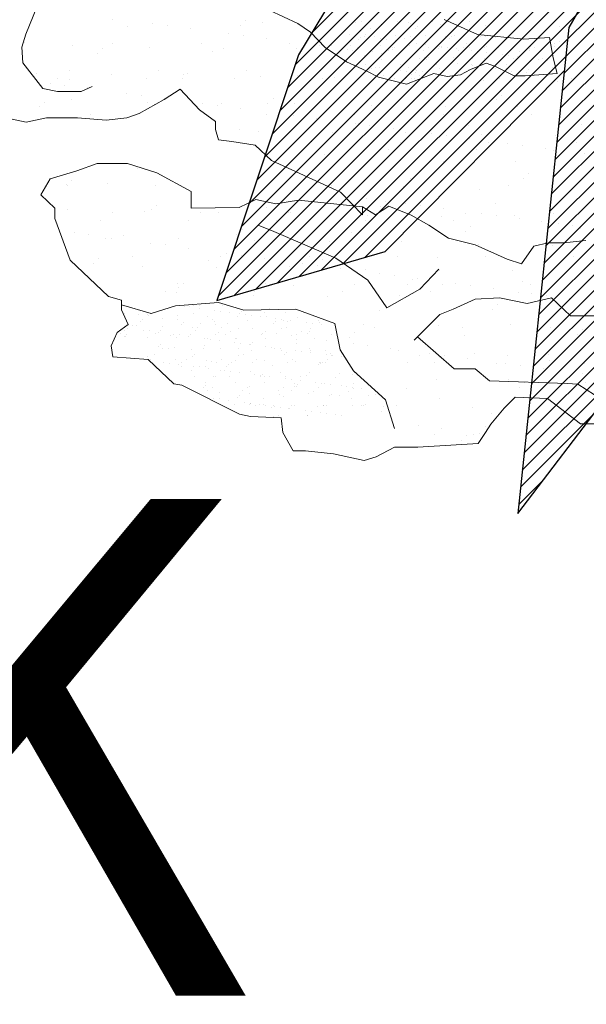
# Model space of a CAD drawing. Units: inches. Extents: x 1986 to 21484, y -1816 to 2016.
# Tile 12 of 85: x 2157 to 2165, y 1860 to 1874. Entities that reach past the tile are written whole.
import ezdxf

# ---------------------------------------------------------------- set-up
doc = ezdxf.new("R2010")
doc.units = ezdxf.units.IN
for name, color, linetype, lineweight in [('A-ANNO-TEXT', 7, 'Continuous', 18), ('L-PLNT', 84, 'Continuous', 13), ('vfolhas', 114, 'Continuous', 5)]:
    doc.layers.add(name, color=color, linetype=linetype, lineweight=lineweight)
doc.layers.add('vfolha2', color=110, linetype='Continuous')
doc.layers.add('vfolhas2', color=102, linetype='Continuous')
doc.styles.get("Standard").update_dxf_attribs({"font": 'arial.ttf'})
pattern_1 = [(45, (-2446.5133113, 50.986076), (-0.004419417382, 0.004419417382), [])]

# ---------------------------------------------------------------- blocks, each defined once
blk = doc.blocks.new('arbusto_PB_verde_grande')
at = {"layer": 'vfolha2'}
h = blk.add_hatch(dxfattribs=at)
h.set_pattern_fill('ANSI31', color=256, scale=0.05, style=0)
h.set_pattern_definition(pattern_1)
h.paths.add_polyline_path([(0.02944, 0.35651), (0.00028, 0.09048), (0.02625, -0.03934), (0.047, 0.06233), (0.06189, 0.09731), (0.09372, 0.26573), (0.09955, 0.43473), (0.08789, 0.61313), (0.0645, 0.72266), (0.04988, 0.6851), (0.0236, 0.51294)])
h.paths.add_polyline_path([(0.30106, 0.43789), (0.14225, 0.24871), (0.26685, 0.30022)])
h.paths.add_polyline_path([(0.37995, 0.22817), (0.23697, 0.15193), (0.18428, 0.09364), (0.11122, 0.04358), (0.02625, -0.03934), (0.28061, 0.04667), (0.36829, 0.07798), (0.46756, 0.11239), (0.61068, 0.19376), (0.71585, 0.27823), (0.55813, 0.25948)])
h.paths.add_polyline_path([(0.56101, -0.29441), (0.72752, -0.32573), (0.59024, -0.2412), (0.42962, -0.15982), (0.02625, -0.03934), (0.14922, -0.14107), (0.18838, -0.16604), (0.41501, -0.24435)])
h.paths.add_polyline_path([(-0.27429, -0.44776), (-0.30352, -0.72628), (-0.23923, -0.64175), (-0.15457, -0.45716), (0.02625, -0.03934), (-0.16328, -0.25376)])
h.paths.add_polyline_path([(-0.51963, -0.24744), (-0.67736, -0.32573), (-0.59558, -0.35072), (-0.40574, -0.32882), (-0.21007, -0.20995), (0.02625, -0.03934), (-0.14874, -0.06595), (-0.31518, -0.09101), (-0.41452, -0.15048)])
h.paths.add_polyline_path([(-0.52546, 0.25007), (-0.70947, 0.24698), (-0.51963, 0.1093), (-0.32979, 0.02167), (-0.07567, -0.0128), (-0.04234, -0.02148), (-0.35024, 0.1312)])
at = {"layer": 'vfolhas'}
h = blk.add_hatch(dxfattribs=at)
h.set_pattern_fill('ANSI31', color=256, scale=0.05, style=0)
h.set_pattern_definition(pattern_1)
h.paths.add_polyline_path([(-0.57219, 0.06233), (-0.7153, 0.10298), (-0.67736, 0.08107), (-0.62769, 0.01536), (-0.56347, -0.04095), (-0.26461, -0.0834), (-0.14874, -0.06595), (-0.10151, -0.05877), (-0.20418, -0.0472), (-0.40279, -0.00339)])
h.paths.add_polyline_path([(-0.56347, -0.04095), (-0.58279, -0.02401), (-0.72992, -0.09726), (-0.4334, -0.1679), (-0.41452, -0.15048), (-0.31518, -0.09101), (-0.26461, -0.0834)])
h.paths.add_polyline_path([(-0.2769, -0.47267), (-0.27429, -0.44776), (-0.16328, -0.25376), (0.02625, -0.03934), (-0.21007, -0.20995), (-0.2672, -0.24466), (-0.36485, -0.35697), (-0.42907, -0.46341), (-0.47586, -0.60425), (-0.37946, -0.57603)])
at = {"layer": 'vfolha2'}
for p, q in [((-0.16328, -0.25376), (-0.27429, -0.44776)), ((-0.27429, -0.44776), (-0.30352, -0.72628)), ((-0.30352, -0.72628), (-0.23923, -0.64175))]:
    blk.add_line(p, q, dxfattribs=at)
at = {"layer": 'vfolhas2'}
for p, q in [((-0.36485, -0.35697), (-0.42907, -0.46341)), ((-0.42907, -0.46341), (-0.47586, -0.60425)), ((-0.37946, -0.57603), (-0.2769, -0.47267)), ((-0.47586, -0.60425), (-0.37946, -0.57603))]:
    blk.add_line(p, q, dxfattribs=at)
blk = doc.blocks.new('PLANT-SHRUB')
for p, q in [((2157.221, 1873.694), (2157.486, 1874.349)), ((2161.057, 1873.846), (2160.649, 1874.033)), ((2158.449, 1873.897), (2158.449, 1873.897)), ((2158.651, 1873.807), (2158.651, 1873.807)), ((2159.005, 1873.85), (2159.005, 1873.85)), ((2159.213, 1873.823), (2159.213, 1873.823)), ((2160.25, 1873.821), (2160.25, 1873.821)), ((2160.324, 1873.889), (2160.324, 1873.889)), ((2160.551, 1873.863), (2160.551, 1873.863)), ((2161.233, 1873.725), (2161.057, 1873.846)), ((2161.597, 1873.849), (2161.597, 1873.849)), ((2161.873, 1873.857), (2161.873, 1873.857)), ((2161.959, 1873.87), (2161.959, 1873.87)), ((2162.228, 1873.838), (2162.228, 1873.838)), ((2162.457, 1873.869), (2162.457, 1873.869)), ((2162.619, 1873.854), (2162.619, 1873.854)), ((2162.637, 1873.84), (2162.637, 1873.84)), ((2162.748, 1873.808), (2162.748, 1873.808)), ((2162.955, 1873.868), (2162.955, 1873.868)), ((2163.069, 1873.825), (2163.069, 1873.825)), ((2163.116, 1873.901), (2163.589, 1873.692)), ((2163.472, 1873.87), (2163.472, 1873.87)), ((2163.699, 1873.815), (2163.699, 1873.815)), ((2164.745, 1873.802), (2164.745, 1873.802)), ((2157.166, 1873.513), (2157.221, 1873.694)), ((2159.538, 1873.78), (2159.538, 1873.78)), ((2160.081, 1873.709), (2160.081, 1873.709)), ((2160.289, 1873.681), (2160.289, 1873.681)), ((2161.442, 1873.505), (2161.233, 1873.725)), ((2161.786, 1873.691), (2161.786, 1873.691)), ((2161.869, 1873.68), (2161.869, 1873.68)), ((2161.999, 1873.663), (2161.999, 1873.663)), ((2162.003, 1873.696), (2162.003, 1873.696)), ((2162.079, 1873.775), (2162.079, 1873.775)), ((2162.14, 1873.667), (2162.14, 1873.667)), ((2162.434, 1873.68), (2162.434, 1873.68)), ((2162.638, 1873.666), (2162.638, 1873.666)), ((2162.718, 1873.781), (2162.718, 1873.781)), ((2162.853, 1873.675), (2162.853, 1873.675)), ((2163.136, 1873.665), (2163.136, 1873.665)), ((2163.228, 1873.667), (2163.228, 1873.667)), ((2163.262, 1873.677), (2163.262, 1873.677)), ((2163.589, 1873.692), (2164.239, 1873.626)), ((2163.634, 1873.664), (2163.634, 1873.664)), ((2163.694, 1873.661), (2163.694, 1873.661)), ((2163.848, 1873.654), (2163.848, 1873.654)), ((2157.18, 1873.29), (2157.166, 1873.513)), ((2157.203, 1873.572), (2157.203, 1873.572)), ((2157.885, 1873.54), (2157.885, 1873.54)), ((2158.447, 1873.57), (2158.447, 1873.57)), ((2159.692, 1873.568), (2159.692, 1873.568)), ((2160.614, 1873.639), (2160.614, 1873.639)), ((2160.937, 1873.565), (2160.937, 1873.565)), ((2161.157, 1873.567), (2161.157, 1873.567)), ((2161.365, 1873.54), (2161.365, 1873.54)), ((2161.525, 1873.538), (2161.525, 1873.538)), ((2161.8, 1873.536), (2161.8, 1873.536)), ((2161.897, 1873.512), (2161.897, 1873.512)), ((2161.91, 1873.621), (2161.91, 1873.621)), ((2161.94, 1873.648), (2161.94, 1873.648)), ((2162.181, 1873.563), (2162.181, 1873.563)), ((2162.216, 1873.635), (2162.216, 1873.635)), ((2162.218, 1873.53), (2162.218, 1873.53)), ((2162.299, 1873.624), (2162.299, 1873.624)), ((2162.395, 1873.512), (2162.395, 1873.512)), ((2162.429, 1873.607), (2162.429, 1873.607)), ((2162.559, 1873.635), (2162.559, 1873.635)), ((2162.627, 1873.532), (2162.627, 1873.532)), ((2162.646, 1873.578), (2162.646, 1873.578)), ((2162.73, 1873.567), (2162.73, 1873.567)), ((2162.86, 1873.55), (2162.86, 1873.55)), ((2163.059, 1873.517), (2163.059, 1873.517)), ((2163.077, 1873.521), (2163.077, 1873.521)), ((2163.199, 1873.64), (2163.199, 1873.64)), ((2163.426, 1873.561), (2163.426, 1873.561)), ((2163.477, 1873.511), (2163.477, 1873.511)), ((2163.709, 1873.527), (2163.709, 1873.527)), ((2163.886, 1873.513), (2163.886, 1873.513)), ((2164.239, 1873.626), (2164.602, 1873.648)), ((2164.329, 1873.514), (2164.329, 1873.514)), ((2164.602, 1873.648), (2164.657, 1873.362)), ((2164.602, 1873.648), (2164.602, 1873.648)), ((2164.671, 1873.559), (2164.671, 1873.559)), ((2164.673, 1873.52), (2164.673, 1873.52)), ((2164.747, 1873.587), (2164.747, 1873.587)), ((2158.229, 1873.421), (2158.229, 1873.421)), ((2158.303, 1873.489), (2158.303, 1873.489)), ((2158.964, 1873.501), (2158.964, 1873.501)), ((2159.852, 1873.457), (2159.852, 1873.457)), ((2160.01, 1873.488), (2160.01, 1873.488)), ((2161.033, 1873.493), (2161.033, 1873.493)), ((2161.739, 1873.307), (2161.442, 1873.505)), ((2161.451, 1873.47), (2161.451, 1873.47)), ((2161.69, 1873.497), (2161.69, 1873.497)), ((2161.751, 1873.475), (2161.751, 1873.475)), ((2161.83, 1873.47), (2161.83, 1873.47)), ((2161.993, 1873.388), (2161.993, 1873.388)), ((2162.112, 1873.454), (2162.112, 1873.454)), ((2162.233, 1873.426), (2162.233, 1873.426)), ((2162.328, 1873.469), (2162.328, 1873.469)), ((2162.391, 1873.48), (2162.391, 1873.48)), ((2162.42, 1873.507), (2162.42, 1873.507)), ((2162.424, 1873.372), (2162.424, 1873.372)), ((2162.441, 1873.398), (2162.441, 1873.398)), ((2162.826, 1873.468), (2162.826, 1873.468)), ((2162.893, 1873.511), (2162.893, 1873.511)), ((2163.04, 1873.494), (2163.04, 1873.494)), ((2163.074, 1873.506), (2163.074, 1873.506)), ((2163.158, 1873.441), (2163.158, 1873.441)), ((2163.16, 1873.51), (2163.16, 1873.51)), ((2163.29, 1873.493), (2163.29, 1873.493)), ((2163.324, 1873.467), (2163.324, 1873.467)), ((2163.391, 1873.51), (2163.391, 1873.51)), ((2163.507, 1873.465), (2163.507, 1873.465)), ((2163.59, 1873.454), (2163.59, 1873.454)), ((2163.68, 1873.5), (2163.68, 1873.5)), ((2163.72, 1873.437), (2163.72, 1873.437)), ((2163.821, 1873.466), (2163.821, 1873.466)), ((2163.889, 1873.509), (2163.889, 1873.509)), ((2163.937, 1873.408), (2163.937, 1873.408)), ((2164.021, 1873.397), (2164.021, 1873.397)), ((2164.151, 1873.38), (2164.151, 1873.38)), ((2164.181, 1873.446), (2164.181, 1873.446)), ((2164.19, 1873.387), (2164.19, 1873.387)), ((2164.318, 1873.498), (2164.318, 1873.498)), ((2164.319, 1873.465), (2164.319, 1873.465)), ((2164.387, 1873.508), (2164.387, 1873.508)), ((2157.458, 1872.928), (2157.18, 1873.29)), ((2162.026, 1873.175), (2161.739, 1873.307)), ((2161.851, 1873.269), (2161.851, 1873.269)), ((2162.011, 1873.267), (2162.011, 1873.267)), ((2162.069, 1873.24), (2162.069, 1873.24)), ((2162.232, 1873.334), (2162.232, 1873.334)), ((2162.509, 1873.266), (2162.509, 1873.266)), ((2162.766, 1873.355), (2162.766, 1873.355)), ((2162.843, 1873.367), (2162.843, 1873.367)), ((2162.871, 1873.34), (2162.871, 1873.34)), ((2162.901, 1873.367), (2162.901, 1873.367)), ((2163.007, 1873.265), (2163.007, 1873.265)), ((2163.252, 1873.369), (2163.252, 1873.369)), ((2163.308, 1873.284), (2163.308, 1873.284)), ((2163.71, 1873.285), (2163.49, 1873.197)), ((2163.505, 1873.264), (2163.505, 1873.264)), ((2163.517, 1873.257), (2163.517, 1873.257)), ((2163.52, 1873.354), (2163.52, 1873.354)), ((2163.684, 1873.353), (2163.684, 1873.353)), ((2163.842, 1873.241), (2163.71, 1873.285)), ((2164.107, 1873.109), (2163.842, 1873.241)), ((2164.002, 1873.263), (2164.002, 1873.263)), ((2164.102, 1873.348), (2164.102, 1873.348)), ((2164.16, 1873.36), (2164.16, 1873.36)), ((2164.368, 1873.351), (2164.368, 1873.351)), ((2164.451, 1873.34), (2164.451, 1873.34)), ((2164.5, 1873.262), (2164.5, 1873.262)), ((2164.511, 1873.35), (2164.511, 1873.35)), ((2164.581, 1873.323), (2164.581, 1873.323)), ((2164.657, 1873.362), (2164.712, 1873.142)), ((2164.67, 1873.246), (2164.67, 1873.246)), ((2157.377, 1873.14), (2157.377, 1873.14)), ((2157.841, 1873.183), (2157.841, 1873.183)), ((2158.424, 1873.127), (2158.424, 1873.127)), ((2159.085, 1873.181), (2159.085, 1873.181)), ((2159.446, 1873.132), (2159.446, 1873.132)), ((2159.504, 1873.138), (2159.504, 1873.138)), ((2160.33, 1873.179), (2160.33, 1873.179)), ((2161.054, 1873.106), (2161.054, 1873.106)), ((2161.575, 1873.177), (2161.575, 1873.177)), ((2162.191, 1873.087), (2162.026, 1873.175)), ((2162.063, 1873.18), (2162.063, 1873.18)), ((2162.092, 1873.207), (2162.092, 1873.207)), ((2162.152, 1873.229), (2162.152, 1873.229)), ((2162.208, 1873.222), (2162.208, 1873.222)), ((2162.266, 1873.111), (2162.266, 1873.111)), ((2162.282, 1873.212), (2162.282, 1873.212)), ((2162.499, 1873.184), (2162.499, 1873.184)), ((2162.582, 1873.173), (2162.582, 1873.173)), ((2162.973, 1873.142), (2162.587, 1872.988)), ((2162.617, 1873.224), (2162.617, 1873.224)), ((2162.653, 1873.12), (2162.653, 1873.12)), ((2162.712, 1873.194), (2162.712, 1873.194)), ((2162.712, 1873.155), (2162.712, 1873.155)), ((2162.726, 1873.187), (2162.726, 1873.187)), ((2162.764, 1873.11), (2162.764, 1873.11)), ((2162.819, 1873.174), (2162.819, 1873.174)), ((2162.929, 1873.127), (2162.929, 1873.127)), ((2162.973, 1873.142), (2162.973, 1873.142)), ((2163.16, 1873.098), (2162.973, 1873.142)), ((2163.049, 1873.209), (2163.049, 1873.209)), ((2163.347, 1873.12), (2163.16, 1873.098)), ((2163.49, 1873.197), (2163.347, 1873.12)), ((2163.352, 1873.2), (2163.352, 1873.2)), ((2163.381, 1873.227), (2163.381, 1873.227)), ((2163.467, 1873.203), (2163.467, 1873.203)), ((2163.841, 1873.214), (2163.841, 1873.214)), ((2164.001, 1873.214), (2164.001, 1873.214)), ((2164.064, 1873.172), (2164.064, 1873.172)), ((2164.261, 1873.109), (2164.107, 1873.109)), ((2164.712, 1873.142), (2164.261, 1873.109)), ((2164.276, 1873.155), (2164.276, 1873.155)), ((2164.308, 1873.19), (2164.308, 1873.19)), ((2164.384, 1873.142), (2164.384, 1873.142)), ((2164.592, 1873.115), (2164.592, 1873.115)), ((2164.641, 1873.219), (2164.641, 1873.219)), ((2164.712, 1873.142), (2164.712, 1873.142)), ((2157.561, 1873.006), (2157.561, 1873.006)), ((2157.672, 1873.076), (2157.672, 1873.076)), ((2157.769, 1872.978), (2157.769, 1872.978)), ((2157.831, 1873.057), (2157.831, 1873.057)), ((2158.155, 1872.956), (2158.002, 1872.886)), ((2158.917, 1873.074), (2158.917, 1873.074)), ((2159.431, 1873.071), (2159.431, 1873.071)), ((2160.161, 1873.071), (2160.161, 1873.071)), ((2160.525, 1873.093), (2160.525, 1873.093)), ((2161.406, 1873.069), (2161.406, 1873.069)), ((2161.572, 1873.079), (2161.572, 1873.079)), ((2162.587, 1872.988), (2162.191, 1873.087)), ((2162.414, 1873.064), (2162.414, 1873.064)), ((2162.544, 1873.04), (2162.544, 1873.04)), ((2162.573, 1873.067), (2162.573, 1873.067)), ((2162.594, 1873.084), (2162.594, 1873.084)), ((2162.651, 1873.067), (2162.651, 1873.067)), ((2162.697, 1873.067), (2162.697, 1873.067)), ((2163.673, 1873.045), (2163.673, 1873.045)), ((2163.895, 1873.065), (2163.895, 1873.065)), ((2164.72, 1873.032), (2164.72, 1873.032)), ((2164.917, 1873.072), (2164.917, 1873.072)), ((2157.458, 1872.928), (2157.458, 1872.928)), ((2157.667, 1872.886), (2157.458, 1872.928)), ((2157.667, 1872.886), (2157.667, 1872.886)), ((2158.002, 1872.886), (2157.667, 1872.886)), ((2158.002, 1872.886), (2158.002, 1872.886)), ((2158.094, 1872.936), (2158.094, 1872.936)), ((2158.637, 1872.864), (2158.637, 1872.864)), ((2158.845, 1872.837), (2158.845, 1872.837)), ((2159.398, 1872.918), (2159.17, 1872.773)), ((2159.667, 1872.628), (2159.398, 1872.918)), ((2163.928, 1872.836), (2163.928, 1872.836)), ((2157.484, 1872.738), (2157.484, 1872.738)), ((2157.859, 1872.77), (2157.859, 1872.77)), ((2159.17, 1872.773), (2158.818, 1872.576)), ((2158.939, 1872.731), (2158.939, 1872.731)), ((2159.033, 1872.706), (2159.033, 1872.706)), ((2159.17, 1872.794), (2159.17, 1872.794)), ((2159.713, 1872.723), (2159.713, 1872.723)), ((2159.921, 1872.695), (2159.921, 1872.695)), ((2159.985, 1872.718), (2159.985, 1872.718)), ((2160.632, 1872.72), (2160.632, 1872.72)), ((2160.706, 1872.787), (2160.706, 1872.787)), ((2161.007, 1872.723), (2161.007, 1872.723)), ((2162.087, 1872.684), (2162.087, 1872.684)), ((2162.255, 1872.755), (2162.255, 1872.755)), ((2163.854, 1872.769), (2163.854, 1872.769)), ((2157.223, 1872.452), (2156.653, 1872.576)), ((2157.41, 1872.671), (2157.41, 1872.671)), ((2158.125, 1872.569), (2158.125, 1872.569)), ((2158.818, 1872.576), (2158.642, 1872.514)), ((2159.895, 1872.463), (2159.667, 1872.628)), ((2160.245, 1872.652), (2160.245, 1872.652)), ((2160.614, 1872.565), (2160.614, 1872.565)), ((2160.788, 1872.581), (2160.788, 1872.581)), ((2160.996, 1872.554), (2160.996, 1872.554)), ((2161.858, 1872.562), (2161.858, 1872.562)), ((2163.103, 1872.56), (2163.103, 1872.56)), ((2163.133, 1872.671), (2163.133, 1872.671)), ((2164.155, 1872.675), (2164.155, 1872.675)), ((2164.348, 1872.558), (2164.348, 1872.558)), ((2157.513, 1872.514), (2157.223, 1872.452)), ((2157.223, 1872.452), (2157.223, 1872.452)), ((2157.948, 1872.514), (2157.513, 1872.514)), ((2158.352, 1872.483), (2157.948, 1872.514)), ((2158.642, 1872.514), (2158.352, 1872.483)), ((2159.895, 1872.349), (2159.895, 1872.463)), ((2161.321, 1872.511), (2161.321, 1872.511)), ((2161.864, 1872.439), (2161.864, 1872.439)), ((2161.907, 1872.437), (2161.907, 1872.437)), ((2162.072, 1872.412), (2162.072, 1872.412)), ((2163.456, 1872.404), (2163.456, 1872.404)), ((2165.056, 1872.418), (2165.056, 1872.418)), ((2159.936, 1872.204), (2159.895, 1872.349)), ((2160.234, 1872.355), (2160.234, 1872.355)), ((2160.5, 1872.323), (2160.5, 1872.323)), ((2161.546, 1872.309), (2161.546, 1872.309)), ((2161.834, 1872.369), (2161.834, 1872.369)), ((2162.397, 1872.369), (2162.397, 1872.369)), ((2162.569, 1872.314), (2162.569, 1872.314)), ((2162.94, 1872.298), (2162.94, 1872.298)), ((2163.148, 1872.27), (2163.148, 1872.27)), ((2163.648, 1872.275), (2163.648, 1872.275)), ((2164.694, 1872.262), (2164.694, 1872.262)), ((2160.123, 1872.183), (2159.936, 1872.204)), ((2160.454, 1872.131), (2160.123, 1872.183)), ((2160.682, 1871.914), (2160.454, 1872.131)), ((2161.252, 1872.176), (2161.252, 1872.176)), ((2162.496, 1872.173), (2162.496, 1872.173)), ((2163.473, 1872.227), (2163.473, 1872.227)), ((2163.741, 1872.171), (2163.741, 1872.171)), ((2164.016, 1872.156), (2164.016, 1872.156)), ((2164.224, 1872.129), (2164.224, 1872.129)), ((2164.986, 1872.169), (2164.986, 1872.169)), ((2161.436, 1872.005), (2161.436, 1872.005)), ((2162.328, 1872.066), (2162.328, 1872.066)), ((2163.035, 1872.018), (2163.035, 1872.018)), ((2163.109, 1872.086), (2163.109, 1872.086)), ((2163.572, 1872.064), (2163.572, 1872.064)), ((2164.549, 1872.086), (2164.549, 1872.086)), ((2164.658, 1872.054), (2164.658, 1872.054)), ((2164.817, 1872.062), (2164.817, 1872.062)), ((2165.092, 1872.014), (2165.092, 1872.014)), ((2157.937, 1871.769), (2158.227, 1871.873)), ((2158.227, 1871.873), (2158.652, 1871.873)), ((2158.227, 1871.873), (2158.227, 1871.873)), ((2158.652, 1871.873), (2159.066, 1871.738)), ((2160.682, 1871.914), (2160.682, 1871.914)), ((2161.656, 1871.469), (2160.682, 1871.914)), ((2162.062, 1871.914), (2162.062, 1871.914)), ((2163.108, 1871.9), (2163.108, 1871.9)), ((2164.13, 1871.905), (2164.13, 1871.905)), ((2157.565, 1871.655), (2157.937, 1871.769)), ((2158.801, 1871.808), (2158.801, 1871.808)), ((2159.066, 1871.738), (2159.553, 1871.479)), ((2164.31, 1871.735), (2164.31, 1871.735)), ((2157.43, 1871.428), (2157.565, 1871.655)), ((2157.792, 1871.569), (2157.792, 1871.569)), ((2157.802, 1871.568), (2157.802, 1871.568)), ((2157.866, 1871.637), (2157.866, 1871.637)), ((2158.373, 1871.586), (2158.373, 1871.586)), ((2162.637, 1871.654), (2162.637, 1871.654)), ((2164.237, 1871.667), (2164.237, 1871.667)), ((2159.046, 1871.566), (2159.046, 1871.566)), ((2159.553, 1871.479), (2159.553, 1871.241)), ((2161.536, 1871.561), (2161.536, 1871.561)), ((2161.966, 1871.148), (2161.656, 1871.469)), ((2162.544, 1871.544), (2162.544, 1871.544)), ((2162.78, 1871.559), (2162.78, 1871.559)), ((2163.623, 1871.505), (2163.623, 1871.505)), ((2164.025, 1871.557), (2164.025, 1871.557)), ((2164.669, 1871.492), (2164.669, 1871.492)), ((2157.43, 1871.428), (2157.43, 1871.428)), ((2157.627, 1871.241), (2157.43, 1871.428)), ((2160.226, 1871.252), (2160.465, 1871.366)), ((2160.465, 1871.366), (2160.744, 1871.303)), ((2160.744, 1871.303), (2161.065, 1871.355)), ((2161.065, 1871.355), (2161.966, 1871.262)), ((2161.704, 1871.426), (2161.704, 1871.426)), ((2162.029, 1871.383), (2162.029, 1871.383)), ((2162.29, 1871.335), (2162.29, 1871.335)), ((2162.571, 1871.311), (2162.571, 1871.311)), ((2163.839, 1871.303), (2163.839, 1871.303)), ((2157.627, 1871.096), (2157.627, 1871.241)), ((2157.809, 1871.23), (2157.809, 1871.23)), ((2158.44, 1871.179), (2158.44, 1871.179)), ((2158.888, 1871.191), (2158.888, 1871.191)), ((2158.994, 1871.219), (2158.994, 1871.219)), ((2159.067, 1871.286), (2159.067, 1871.286)), ((2159.553, 1871.241), (2160.226, 1871.252)), ((2159.684, 1871.177), (2159.684, 1871.177)), ((2159.935, 1871.178), (2159.935, 1871.178)), ((2160.617, 1871.254), (2160.617, 1871.254)), ((2160.929, 1871.175), (2160.929, 1871.175)), ((2160.957, 1871.183), (2160.957, 1871.183)), ((2161.966, 1871.262), (2162.152, 1871.148)), ((2161.966, 1871.262), (2161.966, 1871.148)), ((2162.152, 1871.148), (2162.339, 1871.269)), ((2162.174, 1871.173), (2162.174, 1871.173)), ((2162.216, 1871.268), (2162.216, 1871.268)), ((2162.339, 1871.269), (2162.651, 1871.144)), ((2162.78, 1871.284), (2162.78, 1871.284)), ((2163.104, 1871.241), (2163.104, 1871.241)), ((2163.418, 1871.17), (2163.418, 1871.17)), ((2163.647, 1871.17), (2163.647, 1871.17)), ((2164.663, 1871.168), (2164.663, 1871.168)), ((2157.844, 1870.507), (2157.627, 1871.096)), ((2158.271, 1871.072), (2158.271, 1871.072)), ((2159.516, 1871.07), (2159.516, 1871.07)), ((2160.76, 1871.068), (2160.76, 1871.068)), ((2162.005, 1871.065), (2162.005, 1871.065)), ((2162.036, 1871.144), (2162.036, 1871.144)), ((2162.651, 1871.144), (2162.9, 1871.004)), ((2163.083, 1871.13), (2163.083, 1871.13)), ((2163.25, 1871.063), (2163.25, 1871.063)), ((2163.855, 1871.142), (2163.855, 1871.142)), ((2164.105, 1871.135), (2164.105, 1871.135)), ((2164.18, 1871.1), (2164.18, 1871.1)), ((2164.494, 1871.061), (2164.494, 1871.061)), ((2164.723, 1871.028), (2164.723, 1871.028)), ((2157.9, 1870.892), (2157.9, 1870.892)), ((2160.269, 1870.935), (2160.269, 1870.935)), ((2160.498, 1871.004), (2160.717, 1870.911)), ((2160.717, 1870.911), (2161.59, 1870.537)), ((2161.818, 1870.903), (2161.818, 1870.903)), ((2162.9, 1871.004), (2163.181, 1870.817)), ((2163.417, 1870.917), (2163.417, 1870.917)), ((2163.491, 1870.984), (2163.491, 1870.984)), ((2164.931, 1871.001), (2164.931, 1871.001)), ((2165.04, 1870.952), (2165.04, 1870.952)), ((2158.108, 1870.864), (2158.108, 1870.864)), ((2158.348, 1870.816), (2158.348, 1870.816)), ((2158.433, 1870.821), (2158.433, 1870.821)), ((2158.596, 1870.854), (2158.596, 1870.854)), ((2158.976, 1870.75), (2158.976, 1870.75)), ((2159.37, 1870.821), (2159.37, 1870.821)), ((2160.195, 1870.868), (2160.195, 1870.868)), ((2160.45, 1870.782), (2160.45, 1870.782)), ((2161.496, 1870.769), (2161.496, 1870.769)), ((2162.518, 1870.774), (2162.518, 1870.774)), ((2163.181, 1870.817), (2163.555, 1870.724)), ((2163.181, 1870.817), (2163.181, 1870.817)), ((2163.598, 1870.735), (2163.598, 1870.735)), ((2164.382, 1870.708), (2164.585, 1870.755)), ((2164.585, 1870.755), (2164.803, 1870.755)), ((2164.803, 1870.755), (2165.115, 1870.786)), ((2165.115, 1870.786), (2165.115, 1870.786)), ((2159.184, 1870.723), (2159.184, 1870.723)), ((2159.508, 1870.68), (2159.508, 1870.68)), ((2160.051, 1870.608), (2160.051, 1870.608)), ((2163.555, 1870.724), (2164.008, 1870.521)), ((2164.21, 1870.459), (2164.382, 1870.708)), ((2164.644, 1870.722), (2164.644, 1870.722)), ((2164.692, 1870.634), (2164.692, 1870.634)), ((2157.844, 1870.507), (2157.844, 1870.507)), ((2158.384, 1869.997), (2157.844, 1870.507)), ((2158.175, 1870.468), (2158.175, 1870.468)), ((2158.248, 1870.535), (2158.248, 1870.535)), ((2158.724, 1870.565), (2158.724, 1870.565)), ((2159.797, 1870.503), (2159.797, 1870.503)), ((2159.968, 1870.563), (2159.968, 1870.563)), ((2160.259, 1870.581), (2160.259, 1870.581)), ((2160.584, 1870.538), (2160.584, 1870.538)), ((2161.127, 1870.467), (2161.127, 1870.467)), ((2161.213, 1870.561), (2161.213, 1870.561)), ((2161.397, 1870.517), (2161.397, 1870.517)), ((2161.47, 1870.584), (2161.47, 1870.584)), ((2161.59, 1870.537), (2162.042, 1870.225)), ((2162.458, 1870.558), (2162.458, 1870.558)), ((2163.02, 1870.552), (2163.02, 1870.552)), ((2163.702, 1870.556), (2163.702, 1870.556)), ((2164.008, 1870.521), (2164.21, 1870.459)), ((2164.619, 1870.566), (2164.619, 1870.566)), ((2164.947, 1870.554), (2164.947, 1870.554)), ((2158.863, 1870.421), (2158.863, 1870.421)), ((2159.909, 1870.408), (2159.909, 1870.408)), ((2160.932, 1870.413), (2160.932, 1870.413)), ((2161.335, 1870.439), (2161.335, 1870.439)), ((2161.66, 1870.396), (2161.66, 1870.396)), ((2162.011, 1870.374), (2162.011, 1870.374)), ((2162.203, 1870.325), (2162.203, 1870.325)), ((2162.775, 1870.1), (2163.041, 1870.381)), ((2163.057, 1870.36), (2163.057, 1870.36)), ((2164.08, 1870.365), (2164.08, 1870.365)), ((2159.45, 1870.185), (2159.45, 1870.185)), ((2162.042, 1870.225), (2162.308, 1869.835)), ((2162.411, 1870.298), (2162.411, 1870.298)), ((2162.672, 1870.234), (2162.672, 1870.234)), ((2162.736, 1870.255), (2162.736, 1870.255)), ((2163.279, 1870.183), (2163.279, 1870.183)), ((2164.221, 1870.202), (2164.221, 1870.202)), ((2158.323, 1870.046), (2158.323, 1870.046)), ((2159.193, 1870.069), (2159.193, 1870.069)), ((2159.345, 1870.051), (2159.345, 1870.051)), ((2159.362, 1870.176), (2159.362, 1870.176)), ((2159.376, 1870.117), (2159.376, 1870.117)), ((2160.438, 1870.067), (2160.438, 1870.067)), ((2160.606, 1870.174), (2160.606, 1870.174)), ((2160.999, 1870.152), (2160.999, 1870.152)), ((2161.682, 1870.064), (2161.682, 1870.064)), ((2161.851, 1870.172), (2161.851, 1870.172)), ((2162.308, 1869.835), (2162.775, 1870.1)), ((2162.598, 1870.166), (2162.598, 1870.166)), ((2162.927, 1870.062), (2162.927, 1870.062)), ((2163.095, 1870.17), (2163.095, 1870.17)), ((2163.487, 1870.156), (2163.487, 1870.156)), ((2163.812, 1870.113), (2163.812, 1870.113)), ((2164.172, 1870.06), (2164.172, 1870.06)), ((2164.34, 1870.167), (2164.34, 1870.167)), ((2164.355, 1870.042), (2164.355, 1870.042)), ((2158.384, 1869.997), (2158.384, 1869.997)), ((2158.57, 1869.945), (2158.384, 1869.997)), ((2158.57, 1869.81), (2158.57, 1869.945)), ((2159.329, 1869.866), (2159.937, 1869.913)), ((2159.937, 1869.913), (2160.296, 1869.804)), ((2160.425, 1870.012), (2160.425, 1870.012)), ((2161.471, 1869.999), (2161.471, 1869.999)), ((2162.493, 1870.004), (2162.493, 1870.004)), ((2163.555, 1869.96), (2163.243, 1869.82)), ((2163.898, 1869.976), (2163.555, 1869.96)), ((2163.573, 1869.965), (2163.573, 1869.965)), ((2164.288, 1869.898), (2163.898, 1869.976)), ((2164.631, 1869.976), (2164.288, 1869.898)), ((2164.563, 1870.014), (2164.563, 1870.014)), ((2164.619, 1869.952), (2164.619, 1869.952)), ((2164.897, 1869.726), (2164.631, 1869.976)), ((2164.888, 1869.972), (2164.888, 1869.972)), ((2158.57, 1869.878), (2158.986, 1869.757)), ((2158.663, 1869.603), (2158.57, 1869.81)), ((2158.607, 1869.764), (2158.607, 1869.764)), ((2158.986, 1869.757), (2159.329, 1869.866)), ((2159.451, 1869.859), (2159.451, 1869.859)), ((2159.534, 1869.849), (2159.534, 1869.849)), ((2159.579, 1869.872), (2159.579, 1869.872)), ((2159.664, 1869.831), (2159.664, 1869.831)), ((2159.672, 1869.868), (2159.672, 1869.868)), ((2159.747, 1869.897), (2159.747, 1869.897)), ((2159.881, 1869.803), (2159.881, 1869.803)), ((2159.965, 1869.792), (2159.965, 1869.792)), ((2159.988, 1869.874), (2159.988, 1869.874)), ((2160.095, 1869.775), (2160.095, 1869.775)), ((2160.258, 1869.784), (2160.258, 1869.784)), ((2160.296, 1869.804), (2161.029, 1869.82)), ((2160.296, 1869.804), (2160.296, 1869.804)), ((2160.578, 1869.766), (2160.578, 1869.766)), ((2160.651, 1869.834), (2160.651, 1869.834)), ((2160.877, 1869.771), (2160.877, 1869.771)), ((2161.029, 1869.82), (2161.575, 1869.617)), ((2162.2, 1869.802), (2162.2, 1869.802)), ((2163.243, 1869.82), (2163.056, 1869.742)), ((2163.8, 1869.815), (2163.8, 1869.815)), ((2163.873, 1869.883), (2163.873, 1869.883)), ((2158.815, 1869.736), (2158.815, 1869.736)), ((2158.838, 1869.651), (2158.838, 1869.651)), ((2158.858, 1869.667), (2158.858, 1869.667)), ((2158.939, 1869.737), (2158.939, 1869.737)), ((2158.944, 1869.727), (2158.944, 1869.727)), ((2158.978, 1869.753), (2158.978, 1869.753)), ((2159.14, 1869.693), (2159.14, 1869.693)), ((2159.353, 1869.729), (2159.353, 1869.729)), ((2159.355, 1869.667), (2159.355, 1869.667)), ((2159.588, 1869.751), (2159.588, 1869.751)), ((2159.785, 1869.714), (2159.785, 1869.714)), ((2159.853, 1869.666), (2159.853, 1869.666)), ((2159.884, 1869.638), (2159.884, 1869.638)), ((2160.203, 1869.708), (2160.203, 1869.708)), ((2160.228, 1869.757), (2160.228, 1869.757)), ((2160.312, 1869.746), (2160.312, 1869.746)), ((2160.351, 1869.665), (2160.351, 1869.665)), ((2160.395, 1869.735), (2160.395, 1869.735)), ((2160.525, 1869.718), (2160.525, 1869.718)), ((2160.612, 1869.71), (2160.612, 1869.71)), ((2160.738, 1869.643), (2160.738, 1869.643)), ((2160.742, 1869.69), (2160.742, 1869.69)), ((2160.825, 1869.679), (2160.825, 1869.679)), ((2160.849, 1869.664), (2160.849, 1869.664)), ((2160.907, 1869.642), (2160.907, 1869.642)), ((2160.955, 1869.661), (2160.955, 1869.661)), ((2161.044, 1869.695), (2161.044, 1869.695)), ((2161.172, 1869.633), (2161.172, 1869.633)), ((2161.347, 1869.663), (2161.347, 1869.663)), ((2161.358, 1869.63), (2161.358, 1869.63)), ((2163.056, 1869.742), (2162.697, 1869.383)), ((2163.056, 1869.742), (2163.056, 1869.742)), ((2165.255, 1869.726), (2164.897, 1869.726)), ((2158.425, 1869.303), (2158.508, 1869.49)), ((2158.508, 1869.49), (2158.663, 1869.603)), ((2158.615, 1869.513), (2158.615, 1869.513)), ((2158.656, 1869.55), (2158.656, 1869.55)), ((2158.663, 1869.603), (2158.663, 1869.603)), ((2158.719, 1869.585), (2158.719, 1869.585)), ((2158.78, 1869.591), (2158.78, 1869.591)), ((2158.873, 1869.522), (2158.873, 1869.522)), ((2158.957, 1869.511), (2158.957, 1869.511)), ((2159.087, 1869.494), (2159.087, 1869.494)), ((2159.113, 1869.512), (2159.113, 1869.512)), ((2159.15, 1869.569), (2159.15, 1869.569)), ((2159.42, 1869.597), (2159.42, 1869.597)), ((2159.449, 1869.624), (2159.449, 1869.624)), ((2159.569, 1869.564), (2159.569, 1869.564)), ((2159.611, 1869.511), (2159.611, 1869.511)), ((2159.646, 1869.562), (2159.646, 1869.562)), ((2159.683, 1869.622), (2159.683, 1869.622)), ((2159.891, 1869.595), (2159.891, 1869.595)), ((2159.978, 1869.566), (2159.978, 1869.566)), ((2160.069, 1869.611), (2160.069, 1869.611)), ((2160.108, 1869.51), (2160.108, 1869.51)), ((2160.216, 1869.552), (2160.216, 1869.552)), ((2160.41, 1869.55), (2160.41, 1869.55)), ((2160.606, 1869.509), (2160.606, 1869.509)), ((2160.709, 1869.616), (2160.709, 1869.616)), ((2160.828, 1869.545), (2160.828, 1869.545)), ((2160.89, 1869.56), (2160.89, 1869.56)), ((2161.104, 1869.508), (2161.104, 1869.508)), ((2161.219, 1869.503), (2161.219, 1869.503)), ((2161.237, 1869.547), (2161.237, 1869.547)), ((2161.256, 1869.622), (2161.256, 1869.622)), ((2161.386, 1869.605), (2161.386, 1869.605)), ((2161.575, 1869.617), (2161.652, 1869.243)), ((2161.986, 1869.604), (2161.986, 1869.604)), ((2162.135, 1869.558), (2162.135, 1869.558)), ((2163.032, 1869.59), (2163.032, 1869.59)), ((2163.379, 1869.555), (2163.379, 1869.555)), ((2164.055, 1869.595), (2164.055, 1869.595)), ((2164.624, 1869.553), (2164.624, 1869.553)), ((2165.075, 1869.532), (2165.075, 1869.532)), ((2158.548, 1869.47), (2158.548, 1869.47)), ((2158.612, 1869.437), (2158.612, 1869.437)), ((2158.631, 1869.434), (2158.631, 1869.434)), ((2158.641, 1869.464), (2158.641, 1869.464)), ((2158.934, 1869.419), (2158.934, 1869.419)), ((2159.045, 1869.469), (2159.045, 1869.469)), ((2159.261, 1869.451), (2159.261, 1869.451)), ((2159.304, 1869.465), (2159.304, 1869.465)), ((2159.343, 1869.421), (2159.343, 1869.421)), ((2159.387, 1869.454), (2159.387, 1869.454)), ((2159.517, 1869.437), (2159.517, 1869.437)), ((2159.543, 1869.468), (2159.543, 1869.468)), ((2159.734, 1869.408), (2159.734, 1869.408)), ((2159.775, 1869.406), (2159.775, 1869.406)), ((2159.817, 1869.397), (2159.817, 1869.397)), ((2159.9, 1869.456), (2159.9, 1869.456)), ((2159.93, 1869.483), (2159.93, 1869.483)), ((2159.947, 1869.38), (2159.947, 1869.38)), ((2160.041, 1869.467), (2160.041, 1869.467)), ((2160.164, 1869.352), (2160.164, 1869.352)), ((2160.18, 1869.402), (2160.18, 1869.402)), ((2160.193, 1869.4), (2160.193, 1869.4)), ((2160.539, 1869.466), (2160.539, 1869.466)), ((2160.55, 1869.47), (2160.55, 1869.47)), ((2160.602, 1869.402), (2160.602, 1869.402)), ((2160.759, 1869.48), (2160.759, 1869.48)), ((2160.967, 1869.453), (2160.967, 1869.453)), ((2161.034, 1869.387), (2161.034, 1869.387)), ((2161.037, 1869.465), (2161.037, 1869.465)), ((2161.189, 1869.476), (2161.189, 1869.476)), ((2161.292, 1869.41), (2161.292, 1869.41)), ((2161.453, 1869.381), (2161.453, 1869.381)), ((2161.535, 1869.464), (2161.535, 1869.464)), ((2161.779, 1869.416), (2161.779, 1869.416)), ((2161.853, 1869.483), (2161.853, 1869.483)), ((2162.697, 1869.383), (2162.744, 1869.43)), ((2162.744, 1869.43), (2163.259, 1868.978)), ((2163.402, 1869.451), (2163.402, 1869.451)), ((2165.001, 1869.465), (2165.001, 1869.465)), ((2158.446, 1869.148), (2158.425, 1869.303)), ((2159.092, 1869.296), (2159.092, 1869.296)), ((2159.122, 1869.323), (2159.122, 1869.323)), ((2159.14, 1869.261), (2159.14, 1869.261)), ((2159.226, 1869.266), (2159.226, 1869.266)), ((2159.32, 1869.281), (2159.32, 1869.281)), ((2159.559, 1869.256), (2159.559, 1869.256)), ((2159.724, 1869.265), (2159.724, 1869.265)), ((2159.741, 1869.31), (2159.741, 1869.31)), ((2159.968, 1869.258), (2159.968, 1869.258)), ((2160.222, 1869.264), (2160.222, 1869.264)), ((2160.248, 1869.341), (2160.248, 1869.341)), ((2160.377, 1869.324), (2160.377, 1869.324)), ((2160.381, 1869.316), (2160.381, 1869.316)), ((2160.4, 1869.242), (2160.4, 1869.242)), ((2160.4, 1869.242), (2160.4, 1869.242)), ((2160.41, 1869.343), (2160.41, 1869.343)), ((2160.595, 1869.295), (2160.595, 1869.295)), ((2160.678, 1869.284), (2160.678, 1869.284)), ((2160.72, 1869.264), (2160.72, 1869.264)), ((2160.808, 1869.267), (2160.808, 1869.267)), ((2160.818, 1869.237), (2160.818, 1869.237)), ((2161.025, 1869.238), (2161.025, 1869.238)), ((2161.03, 1869.33), (2161.03, 1869.33)), ((2161.108, 1869.227), (2161.108, 1869.227)), ((2161.218, 1869.263), (2161.218, 1869.263)), ((2161.227, 1869.239), (2161.227, 1869.239)), ((2161.238, 1869.21), (2161.238, 1869.21)), ((2161.446, 1869.229), (2161.446, 1869.229)), ((2161.652, 1869.243), (2161.84, 1868.947)), ((2161.659, 1869.223), (2161.659, 1869.223)), ((2161.835, 1869.339), (2161.835, 1869.339)), ((2162.043, 1869.311), (2162.043, 1869.311)), ((2162.367, 1869.269), (2162.367, 1869.269)), ((2162.468, 1869.234), (2162.468, 1869.234)), ((2158.943, 1869.107), (2158.446, 1869.148)), ((2158.933, 1869.151), (2158.933, 1869.151)), ((2159.305, 1868.765), (2158.943, 1869.107)), ((2158.984, 1869.112), (2158.984, 1869.112)), ((2159.039, 1869.176), (2159.039, 1869.176)), ((2159.156, 1869.07), (2159.156, 1869.07)), ((2159.333, 1869.113), (2159.333, 1869.113)), ((2159.482, 1869.111), (2159.482, 1869.111)), ((2159.573, 1869.156), (2159.573, 1869.156)), ((2159.602, 1869.183), (2159.602, 1869.183)), ((2159.765, 1869.098), (2159.765, 1869.098)), ((2159.832, 1869.083), (2159.832, 1869.083)), ((2159.979, 1869.11), (2159.979, 1869.11)), ((2160.183, 1869.092), (2160.183, 1869.092)), ((2160.222, 1869.17), (2160.222, 1869.17)), ((2160.283, 1869.173), (2160.283, 1869.173)), ((2160.477, 1869.109), (2160.477, 1869.109)), ((2160.592, 1869.094), (2160.592, 1869.094)), ((2160.862, 1869.176), (2160.862, 1869.176)), ((2160.891, 1869.203), (2160.891, 1869.203)), ((2160.975, 1869.108), (2160.975, 1869.108)), ((2161.024, 1869.079), (2161.024, 1869.079)), ((2161.443, 1869.073), (2161.443, 1869.073)), ((2161.455, 1869.182), (2161.455, 1869.182)), ((2161.473, 1869.107), (2161.473, 1869.107)), ((2161.511, 1869.19), (2161.511, 1869.19)), ((2161.528, 1869.171), (2161.528, 1869.171)), ((2161.539, 1869.171), (2161.539, 1869.171)), ((2161.668, 1869.154), (2161.668, 1869.154)), ((2162.773, 1869.169), (2162.773, 1869.169)), ((2162.91, 1869.197), (2162.91, 1869.197)), ((2163.054, 1869.132), (2163.054, 1869.132)), ((2163.118, 1869.17), (2163.118, 1869.17)), ((2163.443, 1869.127), (2163.443, 1869.127)), ((2163.548, 1869.195), (2163.548, 1869.195)), ((2164.017, 1869.167), (2164.017, 1869.167)), ((2164.594, 1869.181), (2164.594, 1869.181)), ((2164.603, 1869.1), (2164.603, 1869.1)), ((2159.239, 1869.059), (2159.239, 1869.059)), ((2159.369, 1869.042), (2159.369, 1869.042)), ((2159.414, 1869.068), (2159.414, 1869.068)), ((2159.414, 1869.01), (2159.414, 1869.01)), ((2159.549, 1868.948), (2159.549, 1868.948)), ((2159.587, 1869.014), (2159.587, 1869.014)), ((2159.67, 1869.003), (2159.67, 1869.003)), ((2159.758, 1869.016), (2159.758, 1869.016)), ((2159.8, 1868.986), (2159.8, 1868.986)), ((2159.912, 1869.067), (2159.912, 1869.067)), ((2159.958, 1868.95), (2159.958, 1868.95)), ((2160.017, 1868.957), (2160.017, 1868.957)), ((2160.053, 1869.016), (2160.053, 1869.016)), ((2160.083, 1869.043), (2160.083, 1869.043)), ((2160.1, 1868.946), (2160.1, 1868.946)), ((2160.115, 1869.066), (2160.115, 1869.066)), ((2160.389, 1868.934), (2160.389, 1868.934)), ((2160.41, 1869.066), (2160.41, 1869.066)), ((2160.702, 1869.03), (2160.702, 1869.03)), ((2160.908, 1869.065), (2160.908, 1869.065)), ((2161.217, 1868.931), (2161.217, 1868.931)), ((2161.342, 1869.035), (2161.342, 1869.035)), ((2161.359, 1869.064), (2161.359, 1869.064)), ((2161.372, 1869.062), (2161.372, 1869.062)), ((2161.381, 1869.051), (2161.381, 1869.051)), ((2161.406, 1869.064), (2161.406, 1869.064)), ((2161.84, 1868.947), (2162.292, 1868.542)), ((2162.604, 1869.061), (2162.604, 1869.061)), ((2162.98, 1869.065), (2162.98, 1869.065)), ((2163.259, 1868.978), (2163.555, 1868.978)), ((2163.259, 1868.978), (2163.259, 1868.978)), ((2163.555, 1868.978), (2163.758, 1868.807)), ((2163.849, 1869.059), (2163.849, 1869.059)), ((2163.986, 1869.055), (2163.986, 1869.055)), ((2164.194, 1869.028), (2164.194, 1869.028)), ((2164.519, 1868.985), (2164.519, 1868.985)), ((2165.093, 1869.057), (2165.093, 1869.057)), ((2159.595, 1868.865), (2159.595, 1868.865)), ((2159.859, 1868.867), (2159.859, 1868.867)), ((2159.894, 1868.87), (2159.894, 1868.87)), ((2160.093, 1868.864), (2160.093, 1868.864)), ((2160.23, 1868.929), (2160.23, 1868.929)), ((2160.447, 1868.9), (2160.447, 1868.9)), ((2160.53, 1868.89), (2160.53, 1868.89)), ((2160.534, 1868.875), (2160.534, 1868.875)), ((2160.563, 1868.902), (2160.563, 1868.902)), ((2160.591, 1868.863), (2160.591, 1868.863)), ((2160.66, 1868.872), (2160.66, 1868.872)), ((2160.808, 1868.929), (2160.808, 1868.929)), ((2160.878, 1868.844), (2160.878, 1868.844)), ((2160.881, 1868.872), (2160.881, 1868.872)), ((2160.961, 1868.833), (2160.961, 1868.833)), ((2161.089, 1868.862), (2161.089, 1868.862)), ((2161.091, 1868.816), (2161.091, 1868.816)), ((2161.183, 1868.89), (2161.183, 1868.89)), ((2161.587, 1868.861), (2161.587, 1868.861)), ((2161.649, 1868.915), (2161.649, 1868.915)), ((2161.823, 1868.895), (2161.823, 1868.895)), ((2161.852, 1868.922), (2161.852, 1868.922)), ((2161.961, 1868.833), (2161.961, 1868.833)), ((2163.007, 1868.82), (2163.007, 1868.82)), ((2163.758, 1868.807), (2164.852, 1868.768)), ((2163.758, 1868.807), (2163.758, 1868.807)), ((2164.03, 1868.825), (2164.03, 1868.825)), ((2165.062, 1868.914), (2165.062, 1868.914)), ((2159.419, 1868.745), (2159.305, 1868.765)), ((2160.231, 1868.339), (2159.419, 1868.745)), ((2159.726, 1868.715), (2159.726, 1868.715)), ((2159.755, 1868.79), (2159.755, 1868.79)), ((2159.755, 1868.742), (2159.755, 1868.742)), ((2159.783, 1868.667), (2159.783, 1868.667)), ((2159.85, 1868.709), (2159.85, 1868.709)), ((2160.173, 1868.784), (2160.173, 1868.784)), ((2160.281, 1868.666), (2160.281, 1868.666)), ((2160.348, 1868.709), (2160.348, 1868.709)), ((2160.375, 1868.73), (2160.375, 1868.73)), ((2160.582, 1868.786), (2160.582, 1868.786)), ((2160.779, 1868.665), (2160.779, 1868.665)), ((2160.846, 1868.708), (2160.846, 1868.708)), ((2160.96, 1868.665), (2160.96, 1868.665)), ((2161.014, 1868.771), (2161.014, 1868.771)), ((2161.014, 1868.735), (2161.014, 1868.735)), ((2161.033, 1868.732), (2161.033, 1868.732)), ((2161.044, 1868.762), (2161.044, 1868.762)), ((2161.276, 1868.664), (2161.276, 1868.664)), ((2161.308, 1868.787), (2161.308, 1868.787)), ((2161.344, 1868.707), (2161.344, 1868.707)), ((2161.391, 1868.776), (2161.391, 1868.776)), ((2161.432, 1868.765), (2161.432, 1868.765)), ((2161.521, 1868.759), (2161.521, 1868.759)), ((2161.664, 1868.749), (2161.664, 1868.749)), ((2161.738, 1868.731), (2161.738, 1868.731)), ((2161.774, 1868.663), (2161.774, 1868.663)), ((2161.821, 1868.72), (2161.821, 1868.72)), ((2161.841, 1868.767), (2161.841, 1868.767)), ((2161.842, 1868.706), (2161.842, 1868.706)), ((2161.951, 1868.702), (2161.951, 1868.702)), ((2162.583, 1868.7), (2162.583, 1868.7)), ((2164.182, 1868.714), (2164.182, 1868.714)), ((2164.256, 1868.781), (2164.256, 1868.781)), ((2164.852, 1868.768), (2165.004, 1868.762)), ((2165.004, 1868.762), (2165.237, 1868.611)), ((2165.109, 1868.786), (2165.109, 1868.786)), ((2159.87, 1868.563), (2159.87, 1868.563)), ((2159.948, 1868.642), (2159.948, 1868.642)), ((2159.953, 1868.552), (2159.953, 1868.552)), ((2160.083, 1868.535), (2160.083, 1868.535)), ((2160.206, 1868.575), (2160.206, 1868.575)), ((2160.236, 1868.602), (2160.236, 1868.602)), ((2160.379, 1868.626), (2160.379, 1868.626)), ((2160.567, 1868.559), (2160.567, 1868.559)), ((2160.798, 1868.621), (2160.798, 1868.621)), ((2160.855, 1868.589), (2160.855, 1868.589)), ((2161.207, 1868.623), (2161.207, 1868.623)), ((2161.495, 1868.595), (2161.495, 1868.595)), ((2161.525, 1868.622), (2161.525, 1868.622)), ((2161.639, 1868.607), (2161.639, 1868.607)), ((2161.812, 1868.557), (2161.812, 1868.557)), ((2162.057, 1868.602), (2162.057, 1868.602)), ((2162.144, 1868.609), (2162.144, 1868.609)), ((2162.292, 1868.542), (2162.417, 1868.137)), ((2163.057, 1868.555), (2163.057, 1868.555)), ((2164.117, 1868.578), (2163.962, 1868.423)), ((2164.117, 1868.578), (2164.117, 1868.578)), ((2164.573, 1868.557), (2164.117, 1868.578)), ((2164.301, 1868.552), (2164.301, 1868.552)), ((2164.573, 1868.557), (2164.573, 1868.557)), ((2165.041, 1868.204), (2164.573, 1868.557)), ((2160.163, 1868.476), (2160.163, 1868.476)), ((2160.3, 1868.506), (2160.3, 1868.506)), ((2160.374, 1868.472), (2160.374, 1868.472)), ((2160.383, 1868.495), (2160.383, 1868.495)), ((2160.39, 1868.494), (2160.39, 1868.494)), ((2160.462, 1868.463), (2160.462, 1868.463)), ((2160.513, 1868.478), (2160.513, 1868.478)), ((2160.572, 1868.478), (2160.572, 1868.478)), ((2160.598, 1868.467), (2160.598, 1868.467)), ((2160.687, 1868.435), (2160.687, 1868.435)), ((2160.716, 1868.462), (2160.716, 1868.462)), ((2160.73, 1868.449), (2160.73, 1868.449)), ((2160.813, 1868.438), (2160.813, 1868.438)), ((2160.923, 1868.424), (2160.923, 1868.424)), ((2160.943, 1868.421), (2160.943, 1868.421)), ((2160.96, 1868.462), (2160.96, 1868.462)), ((2161.004, 1868.463), (2161.004, 1868.463)), ((2161.16, 1868.393), (2161.16, 1868.393)), ((2161.244, 1868.382), (2161.244, 1868.382)), ((2161.336, 1868.449), (2161.336, 1868.449)), ((2161.421, 1868.459), (2161.421, 1868.459)), ((2161.422, 1868.457), (2161.422, 1868.457)), ((2161.457, 1868.461), (2161.457, 1868.461)), ((2161.831, 1868.459), (2161.831, 1868.459)), ((2161.955, 1868.46), (2161.955, 1868.46)), ((2161.976, 1868.454), (2161.976, 1868.454)), ((2162.005, 1868.481), (2162.005, 1868.481)), ((2162.235, 1868.382), (2162.235, 1868.382)), ((2162.263, 1868.444), (2162.263, 1868.444)), ((2162.443, 1868.464), (2162.443, 1868.464)), ((2163.522, 1868.425), (2163.522, 1868.425)), ((2163.962, 1868.423), (2163.775, 1868.195)), ((2163.962, 1868.423), (2163.962, 1868.423)), ((2160.386, 1868.307), (2160.231, 1868.339)), ((2160.821, 1868.287), (2160.386, 1868.307)), ((2160.717, 1868.307), (2160.717, 1868.307)), ((2160.788, 1868.313), (2160.788, 1868.313)), ((2160.842, 1868.08), (2160.821, 1868.287)), ((2161.197, 1868.321), (2161.197, 1868.321)), ((2161.197, 1868.315), (2161.197, 1868.315)), ((2161.374, 1868.365), (2161.374, 1868.365)), ((2161.466, 1868.352), (2161.466, 1868.352)), ((2161.591, 1868.336), (2161.591, 1868.336)), ((2161.674, 1868.325), (2161.674, 1868.325)), ((2161.674, 1868.325), (2161.674, 1868.325)), ((2163.784, 1868.349), (2163.784, 1868.349)), ((2162.75, 1868.183), (2162.75, 1868.183)), ((2163.075, 1868.141), (2163.075, 1868.141)), ((2163.695, 1868.166), (2163.695, 1868.166)), ((2163.775, 1868.195), (2163.703, 1868.081)), ((2165.041, 1868.204), (2165.041, 1868.204)), ((2165.311, 1868.204), (2165.041, 1868.204)), ((2160.987, 1867.821), (2160.842, 1868.08)), ((2162.982, 1868.05), (2162.982, 1868.05)), ((2163.363, 1867.963), (2163.363, 1867.963)), ((2163.436, 1868.031), (2163.436, 1868.031)), ((2163.526, 1868.058), (2163.526, 1868.058)), ((2163.703, 1868.081), (2163.599, 1867.926)), ((2163.618, 1868.069), (2163.618, 1868.069)), ((2163.703, 1868.081), (2163.703, 1868.081)), ((2161.163, 1867.821), (2160.987, 1867.821)), ((2161.557, 1867.78), (2161.163, 1867.821)), ((2162.416, 1867.873), (2162.158, 1867.738)), ((2162.748, 1867.873), (2162.416, 1867.873)), ((2163.599, 1867.926), (2162.748, 1867.873)), ((2162.748, 1867.873), (2162.748, 1867.873)), ((2161.992, 1867.687), (2161.557, 1867.78)), ((2162.158, 1867.738), (2161.992, 1867.687))]:
    blk.add_line(p, q)

msp = doc.modelspace()

# ---------------------------------------------------------------- block references
at = {"layer": 'L-PLNT'}
msp.add_blockref('PLANT-SHRUB', (0, 0), dxfattribs=at)
at = {"layer": 'L-PLNT', "xscale": 24.60366729364114, "yscale": 24.60366729364114, "zscale": 24.60366729364114}
msp.add_blockref('arbusto_PB_verde_grande', (2171.623, 1884.805), dxfattribs=at)

# ---------------------------------------------------------------- texts
at = {"layer": 'A-ANNO-TEXT', "insert": (2108.883, 1867.143), "char_height": 7, "attachment_point": 1}
msp.add_mtext_dynamic_manual_height_columns("{\\fTimes New Roman|b0|i0|c0|p18;4' SETBACK}", width=105.61268, gutter_width=12.5, heights=[0], dxfattribs=at)

doc.saveas('drawing.dxf')
